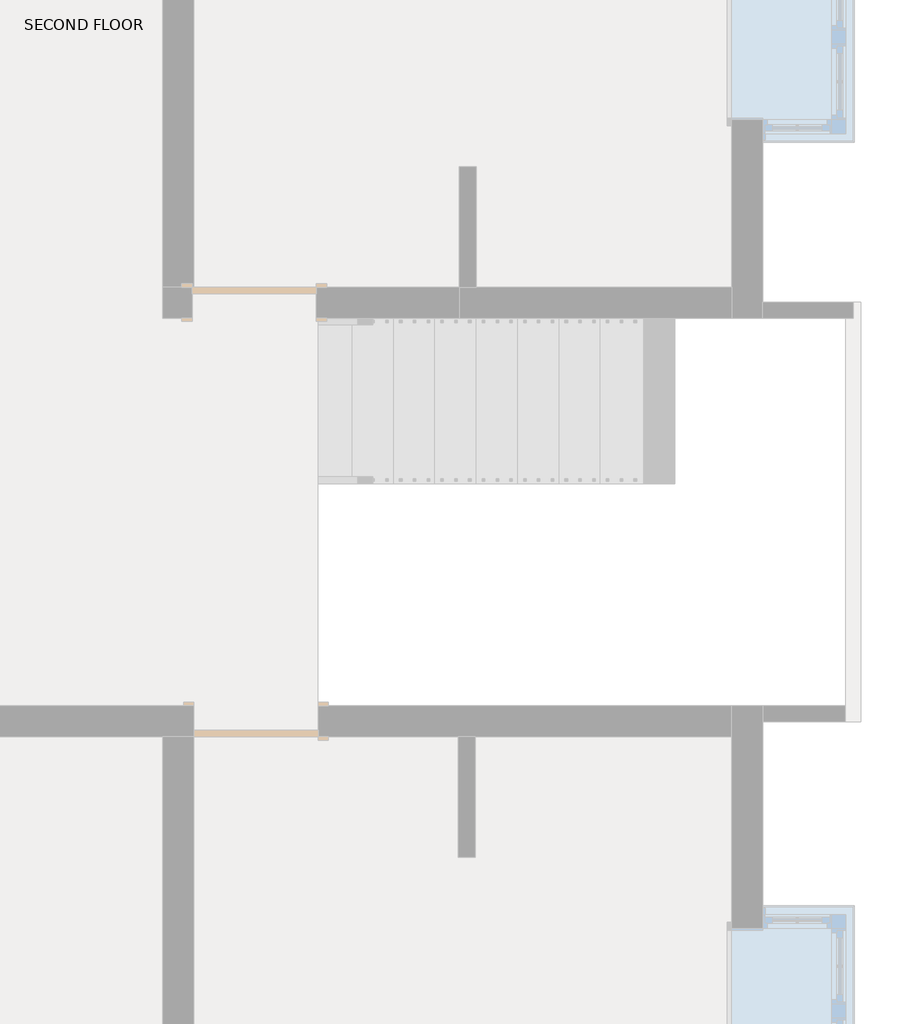
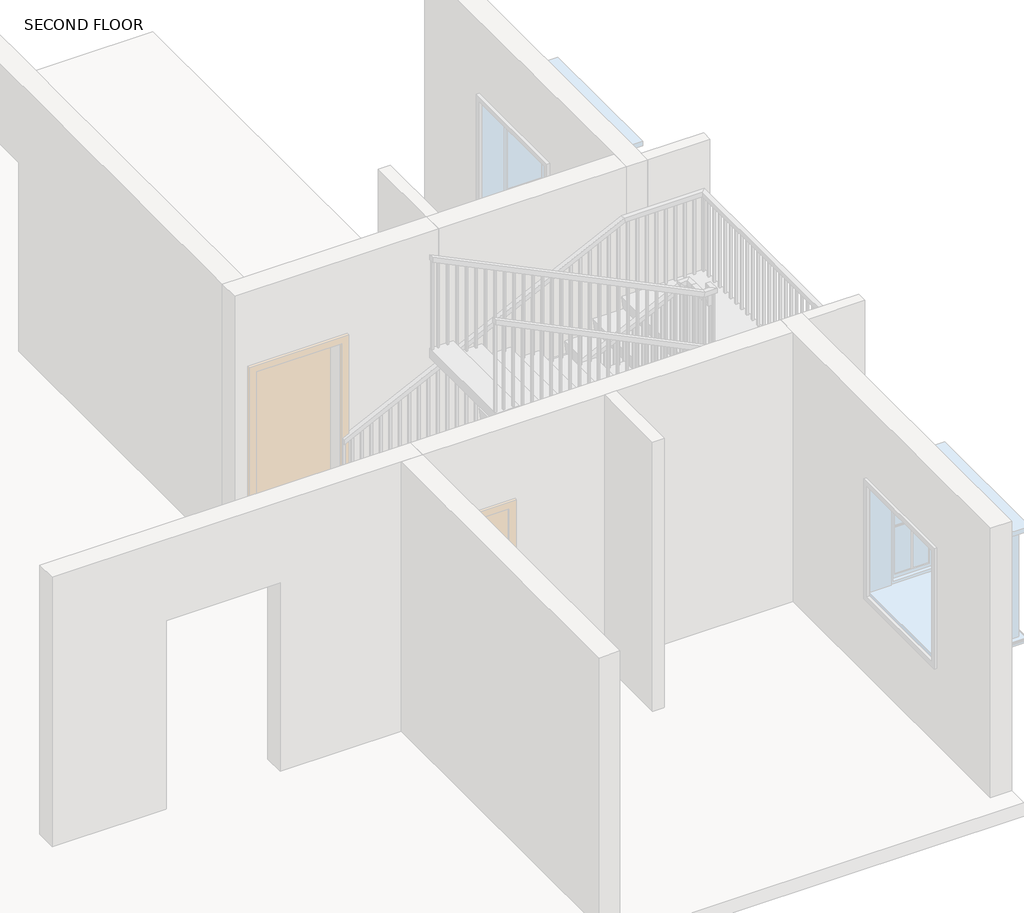
# One storey, part 5 of 6: 1 railing.
"""IFC4 building model written with IfcOpenShell, lengths in millimetres."""

from ifc_helpers import new_model, si_unit, frame, origin, place, context, project, spatial, polyline, outline, extrude, faceted_brep, element, save

model = new_model("IFC4")

# Units and contexts
model_context = context("Model", 3, world=origin())
ifc_project = project(units=[si_unit("LENGTHUNIT", "METRE", prefix="MILLI")], contexts=[model_context])

# Site, building, storey
site = spatial("IfcSite", under=ifc_project)
building = spatial("IfcBuilding", under=site)
storey = spatial("IfcBuildingStorey", under=building, Name="SECOND FLOOR", Elevation=6400.8)

# Railing
placement = place(None, origin())
element("IfcRailing", 1, ObjectType="Handrail - Rectangular", at=placement, inside=storey, context=model_context, shape_type="SolidModel", body=[
    faceted_brep([(3126.2584916, 220.733346, 7460.6727273), (3126.2584916, 220.733346, 7404.1956113), (3126.2584916, 169.933346, 7404.1956113), (3126.2584916, 169.933346, 7460.6727273), (6120.7829507, 220.733346, 8915.4), (6132.4691705, 220.733346, 8864.6), (6132.4691705, 169.933346, 8864.6), (6120.7829507, 169.933346, 8915.4), (7009.1350459, 220.733346, 8915.4), (7009.1350459, 220.733346, 8864.6), (6958.3350459, 169.933346, 8864.6), (6958.3350459, 169.933346, 8915.4), (7009.1350459, -2636.766654, 8915.4), (7009.1350459, -2636.766654, 8864.6), (6958.3350459, -2585.966654, 8864.6), (6958.3350459, -2585.966654, 8915.4), (6420.2353966, -2636.766654, 8915.4), (6408.5491768, -2636.766654, 8864.6), (6408.5491768, -2585.966654, 8864.6), (6420.2353966, -2585.966654, 8915.4), (3126.2584916, -2636.766654, 10515.6), (3126.2584916, -2585.966654, 10515.6), (3126.2584916, -2585.966654, 10459.122884), (3126.2584916, -2636.766654, 10459.122884)], [[[0, 1, 2, 3]], [[1, 0, 4, 5]], [[2, 1, 5, 6]], [[3, 2, 6, 7]], [[0, 3, 7, 4]], [[5, 4, 8, 9]], [[6, 5, 9, 10]], [[7, 6, 10, 11]], [[4, 7, 11, 8]], [[9, 8, 12, 13]], [[10, 9, 13, 14]], [[11, 10, 14, 15]], [[8, 11, 15, 12]], [[13, 12, 16, 17]], [[14, 13, 17, 18]], [[15, 14, 18, 19]], [[12, 15, 19, 16]], [[20, 21, 22, 23]], [[17, 16, 20, 23]], [[18, 17, 23, 22]], [[19, 18, 22, 21]], [[16, 19, 21, 20]]]),
    extrude(outline(polyline([(10416.0077556, 3215.0100459), (9455.7272727, 3215.0100459), (9455.7272727, 3234.0600459), (10406.7533465, 3234.0600459), (10416.0077556, 3215.0100459)])), frame((0.0, -2620.891654, 0.0), z_axis=(0.0, 1.0, 0.0), x_axis=(0.0, 0.0, 1.0)), (0.0, 0.0, 1.0), 19.05),
    extrude(outline(polyline([(10366.6509068, 3316.6100459), (9455.7272727, 3316.6100459), (9455.7272727, 3335.6600459), (10357.3964977, 3335.6600459), (10366.6509068, 3316.6100459)])), frame((0.0, -2620.891654, 0.0), z_axis=(0.0, 1.0, 0.0), x_axis=(0.0, 0.0, 1.0)), (0.0, 0.0, 1.0), 19.05),
    extrude(outline(polyline([(10317.294058, 3418.2100459), (9310.2545455, 3418.2100459), (9310.2545455, 3437.2600459), (10308.0396489, 3437.2600459), (10317.294058, 3418.2100459)])), frame((0.0, -2620.891654, 0.0), z_axis=(0.0, 1.0, 0.0), x_axis=(0.0, 0.0, 1.0)), (0.0, 0.0, 1.0), 19.05),
    extrude(outline(polyline([(10267.9372093, 3519.8100459), (9310.2545455, 3519.8100459), (9310.2545455, 3538.8600459), (10258.6828001, 3538.8600459), (10267.9372093, 3519.8100459)])), frame((0.0, -2620.891654, 0.0), z_axis=(0.0, 1.0, 0.0), x_axis=(0.0, 0.0, 1.0)), (0.0, 0.0, 1.0), 19.05),
    extrude(outline(polyline([(10218.5803605, 3621.4100459), (9310.2545455, 3621.4100459), (9310.2545455, 3640.4600459), (10209.3259513, 3640.4600459), (10218.5803605, 3621.4100459)])), frame((0.0, -2620.891654, 0.0), z_axis=(0.0, 1.0, 0.0), x_axis=(0.0, 0.0, 1.0)), (0.0, 0.0, 1.0), 19.05),
    extrude(outline(polyline([(10169.2235117, 3723.0100459), (9164.7818182, 3723.0100459), (9164.7818182, 3742.0600459), (10159.9691025, 3742.0600459), (10169.2235117, 3723.0100459)])), frame((0.0, -2620.891654, 0.0), z_axis=(0.0, 1.0, 0.0), x_axis=(0.0, 0.0, 1.0)), (0.0, 0.0, 1.0), 19.05),
    extrude(outline(polyline([(10119.8666629, 3824.6100459), (9164.7818182, 3824.6100459), (9164.7818182, 3843.6600459), (10110.6122538, 3843.6600459), (10119.8666629, 3824.6100459)])), frame((0.0, -2620.891654, 0.0), z_axis=(0.0, 1.0, 0.0), x_axis=(0.0, 0.0, 1.0)), (0.0, 0.0, 1.0), 19.05),
    extrude(outline(polyline([(10070.5098141, 3926.2100459), (9164.7818182, 3926.2100459), (9164.7818182, 3945.2600459), (10061.255405, 3945.2600459), (10070.5098141, 3926.2100459)])), frame((0.0, -2620.891654, 0.0), z_axis=(0.0, 1.0, 0.0), x_axis=(0.0, 0.0, 1.0)), (0.0, 0.0, 1.0), 19.05),
    extrude(outline(polyline([(10021.1529653, 4027.8100459), (9019.3090909, 4027.8100459), (9019.3090909, 4046.8600459), (10011.8985562, 4046.8600459), (10021.1529653, 4027.8100459)])), frame((0.0, -2620.891654, 0.0), z_axis=(0.0, 1.0, 0.0), x_axis=(0.0, 0.0, 1.0)), (0.0, 0.0, 1.0), 19.05),
    extrude(outline(polyline([(9971.7961165, 4129.4100459), (9019.3090909, 4129.4100459), (9019.3090909, 4148.4600459), (9962.5417074, 4148.4600459), (9971.7961165, 4129.4100459)])), frame((0.0, -2620.891654, 0.0), z_axis=(0.0, 1.0, 0.0), x_axis=(0.0, 0.0, 1.0)), (0.0, 0.0, 1.0), 19.05),
    extrude(outline(polyline([(9922.4392678, 4231.0100459), (9019.3090909, 4231.0100459), (9019.3090909, 4250.0600459), (9913.1848586, 4250.0600459), (9922.4392678, 4231.0100459)])), frame((0.0, -2620.891654, 0.0), z_axis=(0.0, 1.0, 0.0), x_axis=(0.0, 0.0, 1.0)), (0.0, 0.0, 1.0), 19.05),
    extrude(outline(polyline([(9873.082419, 4332.6100459), (8873.8363636, 4332.6100459), (8873.8363636, 4351.6600459), (9863.8280098, 4351.6600459), (9873.082419, 4332.6100459)])), frame((0.0, -2620.891654, 0.0), z_axis=(0.0, 1.0, 0.0), x_axis=(0.0, 0.0, 1.0)), (0.0, 0.0, 1.0), 19.05),
    extrude(outline(polyline([(9823.7255702, 4434.2100459), (8873.8363636, 4434.2100459), (8873.8363636, 4453.2600459), (9814.471161, 4453.2600459), (9823.7255702, 4434.2100459)])), frame((0.0, -2620.891654, 0.0), z_axis=(0.0, 1.0, 0.0), x_axis=(0.0, 0.0, 1.0)), (0.0, 0.0, 1.0), 19.05),
    extrude(outline(polyline([(9774.3687214, 4535.8100459), (8873.8363636, 4535.8100459), (8873.8363636, 4554.8600459), (9765.1143123, 4554.8600459), (9774.3687214, 4535.8100459)])), frame((0.0, -2620.891654, 0.0), z_axis=(0.0, 1.0, 0.0), x_axis=(0.0, 0.0, 1.0)), (0.0, 0.0, 1.0), 19.05),
    extrude(outline(polyline([(9725.0118726, 4637.4100459), (8728.3636364, 4637.4100459), (8728.3636364, 4656.4600459), (9715.7574635, 4656.4600459), (9725.0118726, 4637.4100459)])), frame((0.0, -2620.891654, 0.0), z_axis=(0.0, 1.0, 0.0), x_axis=(0.0, 0.0, 1.0)), (0.0, 0.0, 1.0), 19.05),
    extrude(outline(polyline([(9675.6550238, 4739.0100459), (8728.3636364, 4739.0100459), (8728.3636364, 4758.0600459), (9666.4006147, 4758.0600459), (9675.6550238, 4739.0100459)])), frame((0.0, -2620.891654, 0.0), z_axis=(0.0, 1.0, 0.0), x_axis=(0.0, 0.0, 1.0)), (0.0, 0.0, 1.0), 19.05),
    extrude(outline(polyline([(9626.2981751, 4840.6100459), (8728.3636364, 4840.6100459), (8728.3636364, 4859.6600459), (9617.0437659, 4859.6600459), (9626.2981751, 4840.6100459)])), frame((0.0, -2620.891654, 0.0), z_axis=(0.0, 1.0, 0.0), x_axis=(0.0, 0.0, 1.0)), (0.0, 0.0, 1.0), 19.05),
    extrude(outline(polyline([(9576.9413263, 4942.2100459), (8582.8909091, 4942.2100459), (8582.8909091, 4961.2600459), (9567.6869171, 4961.2600459), (9576.9413263, 4942.2100459)])), frame((0.0, -2620.891654, 0.0), z_axis=(0.0, 1.0, 0.0), x_axis=(0.0, 0.0, 1.0)), (0.0, 0.0, 1.0), 19.05),
    extrude(outline(polyline([(9527.5844775, 5043.8100459), (8582.8909091, 5043.8100459), (8582.8909091, 5062.8600459), (9518.3300683, 5062.8600459), (9527.5844775, 5043.8100459)])), frame((0.0, -2620.891654, 0.0), z_axis=(0.0, 1.0, 0.0), x_axis=(0.0, 0.0, 1.0)), (0.0, 0.0, 1.0), 19.05),
    extrude(outline(polyline([(9478.2276287, 5145.4100459), (8582.8909091, 5145.4100459), (8582.8909091, 5164.4600459), (9468.9732196, 5164.4600459), (9478.2276287, 5145.4100459)])), frame((0.0, -2620.891654, 0.0), z_axis=(0.0, 1.0, 0.0), x_axis=(0.0, 0.0, 1.0)), (0.0, 0.0, 1.0), 19.05),
    extrude(outline(polyline([(9428.8707799, 5247.0100459), (8437.4181818, 5247.0100459), (8437.4181818, 5266.0600459), (9419.6163708, 5266.0600459), (9428.8707799, 5247.0100459)])), frame((0.0, -2620.891654, 0.0), z_axis=(0.0, 1.0, 0.0), x_axis=(0.0, 0.0, 1.0)), (0.0, 0.0, 1.0), 19.05),
    extrude(outline(polyline([(9379.5139311, 5348.6100459), (8437.4181818, 5348.6100459), (8437.4181818, 5367.6600459), (9370.259522, 5367.6600459), (9379.5139311, 5348.6100459)])), frame((0.0, -2620.891654, 0.0), z_axis=(0.0, 1.0, 0.0), x_axis=(0.0, 0.0, 1.0)), (0.0, 0.0, 1.0), 19.05),
    extrude(outline(polyline([(9330.1570823, 5450.2100459), (8437.4181818, 5450.2100459), (8437.4181818, 5469.2600459), (9320.9026732, 5469.2600459), (9330.1570823, 5450.2100459)])), frame((0.0, -2620.891654, 0.0), z_axis=(0.0, 1.0, 0.0), x_axis=(0.0, 0.0, 1.0)), (0.0, 0.0, 1.0), 19.05),
    extrude(outline(polyline([(9280.8002336, 5551.8100459), (8291.9454545, 5551.8100459), (8291.9454545, 5570.8600459), (9271.5458244, 5570.8600459), (9280.8002336, 5551.8100459)])), frame((0.0, -2620.891654, 0.0), z_axis=(0.0, 1.0, 0.0), x_axis=(0.0, 0.0, 1.0)), (0.0, 0.0, 1.0), 19.05),
    extrude(outline(polyline([(9231.4433848, 5653.4100459), (8291.9454545, 5653.4100459), (8291.9454545, 5672.4600459), (9222.1889756, 5672.4600459), (9231.4433848, 5653.4100459)])), frame((0.0, -2620.891654, 0.0), z_axis=(0.0, 1.0, 0.0), x_axis=(0.0, 0.0, 1.0)), (0.0, 0.0, 1.0), 19.05),
    extrude(outline(polyline([(9182.086536, 5755.0100459), (8291.9454545, 5755.0100459), (8291.9454545, 5774.0600459), (9172.8321268, 5774.0600459), (9182.086536, 5755.0100459)])), frame((0.0, -2620.891654, 0.0), z_axis=(0.0, 1.0, 0.0), x_axis=(0.0, 0.0, 1.0)), (0.0, 0.0, 1.0), 19.05),
    extrude(outline(polyline([(9132.7296872, 5856.6100459), (8146.4727273, 5856.6100459), (8146.4727273, 5875.6600459), (9123.4752781, 5875.6600459), (9132.7296872, 5856.6100459)])), frame((0.0, -2620.891654, 0.0), z_axis=(0.0, 1.0, 0.0), x_axis=(0.0, 0.0, 1.0)), (0.0, 0.0, 1.0), 19.05),
    extrude(outline(polyline([(9083.3728384, 5958.2100459), (8146.4727273, 5958.2100459), (8146.4727273, 5977.2600459), (9074.1184293, 5977.2600459), (9083.3728384, 5958.2100459)])), frame((0.0, -2620.891654, 0.0), z_axis=(0.0, 1.0, 0.0), x_axis=(0.0, 0.0, 1.0)), (0.0, 0.0, 1.0), 19.05),
    extrude(outline(polyline([(9034.0159896, 6059.8100459), (8146.4727273, 6059.8100459), (8146.4727273, 6078.8600459), (9024.7615805, 6078.8600459), (9034.0159896, 6059.8100459)])), frame((0.0, -2620.891654, 0.0), z_axis=(0.0, 1.0, 0.0), x_axis=(0.0, 0.0, 1.0)), (0.0, 0.0, 1.0), 19.05),
    extrude(outline(polyline([(8984.6591409, 6161.4100459), (8001.0, 6161.4100459), (8001.0, 6180.4600459), (8975.4047317, 6180.4600459), (8984.6591409, 6161.4100459)])), frame((0.0, -2620.891654, 0.0), z_axis=(0.0, 1.0, 0.0), x_axis=(0.0, 0.0, 1.0)), (0.0, 0.0, 1.0), 19.05),
    extrude(outline(polyline([(8935.3022921, 6263.0100459), (8001.0, 6263.0100459), (8001.0, 6282.0600459), (8926.0478829, 6282.0600459), (8935.3022921, 6263.0100459)])), frame((0.0, -2620.891654, 0.0), z_axis=(0.0, 1.0, 0.0), x_axis=(0.0, 0.0, 1.0)), (0.0, 0.0, 1.0), 19.05),
    extrude(outline(polyline([(8885.9454433, 6364.6100459), (8001.0, 6364.6100459), (8001.0, 6383.6600459), (8876.6910341, 6383.6600459), (8885.9454433, 6364.6100459)])), frame((0.0, -2620.891654, 0.0), z_axis=(0.0, 1.0, 0.0), x_axis=(0.0, 0.0, 1.0)), (0.0, 0.0, 1.0), 19.05),
    extrude(outline(polyline([(6485.2600459, -2620.891654), (6466.2100459, -2620.891654), (6466.2100459, -2601.841654), (6485.2600459, -2601.841654), (6485.2600459, -2620.891654)])), frame((0.0, 0.0, 8001.0), z_axis=(0.0, 0.0, 1.0), x_axis=(1.0, 0.0, 0.0)), (0.0, 0.0, 1.0), 863.6),
    extrude(outline(polyline([(6586.8600459, -2620.891654), (6567.8100459, -2620.891654), (6567.8100459, -2601.841654), (6586.8600459, -2601.841654), (6586.8600459, -2620.891654)])), frame((0.0, 0.0, 8001.0), z_axis=(0.0, 0.0, 1.0), x_axis=(1.0, 0.0, 0.0)), (0.0, 0.0, 1.0), 863.6),
    extrude(outline(polyline([(6688.4600459, -2620.891654), (6669.4100459, -2620.891654), (6669.4100459, -2601.841654), (6688.4600459, -2601.841654), (6688.4600459, -2620.891654)])), frame((0.0, 0.0, 8001.0), z_axis=(0.0, 0.0, 1.0), x_axis=(1.0, 0.0, 0.0)), (0.0, 0.0, 1.0), 863.6),
    extrude(outline(polyline([(6790.0600459, -2620.891654), (6771.0100459, -2620.891654), (6771.0100459, -2601.841654), (6790.0600459, -2601.841654), (6790.0600459, -2620.891654)])), frame((0.0, 0.0, 8001.0), z_axis=(0.0, 0.0, 1.0), x_axis=(1.0, 0.0, 0.0)), (0.0, 0.0, 1.0), 863.6),
    extrude(outline(polyline([(6891.6600459, -2620.891654), (6872.6100459, -2620.891654), (6872.6100459, -2601.841654), (6891.6600459, -2601.841654), (6891.6600459, -2620.891654)])), frame((0.0, 0.0, 8001.0), z_axis=(0.0, 0.0, 1.0), x_axis=(1.0, 0.0, 0.0)), (0.0, 0.0, 1.0), 863.6),
    extrude(outline(polyline([(6993.2600459, -2538.341654), (6993.2600459, -2557.391654), (6974.2100459, -2557.391654), (6974.2100459, -2538.341654), (6993.2600459, -2538.341654)])), frame((0.0, 0.0, 8001.0), z_axis=(0.0, 0.0, 1.0), x_axis=(1.0, 0.0, 0.0)), (0.0, 0.0, 1.0), 863.6),
    extrude(outline(polyline([(6993.2600459, -2436.741654), (6993.2600459, -2455.791654), (6974.2100459, -2455.791654), (6974.2100459, -2436.741654), (6993.2600459, -2436.741654)])), frame((0.0, 0.0, 8001.0), z_axis=(0.0, 0.0, 1.0), x_axis=(1.0, 0.0, 0.0)), (0.0, 0.0, 1.0), 863.6),
    extrude(outline(polyline([(6993.2600459, -2335.141654), (6993.2600459, -2354.191654), (6974.2100459, -2354.191654), (6974.2100459, -2335.141654), (6993.2600459, -2335.141654)])), frame((0.0, 0.0, 8001.0), z_axis=(0.0, 0.0, 1.0), x_axis=(1.0, 0.0, 0.0)), (0.0, 0.0, 1.0), 863.6),
    extrude(outline(polyline([(6993.2600459, -2233.541654), (6993.2600459, -2252.591654), (6974.2100459, -2252.591654), (6974.2100459, -2233.541654), (6993.2600459, -2233.541654)])), frame((0.0, 0.0, 8001.0), z_axis=(0.0, 0.0, 1.0), x_axis=(1.0, 0.0, 0.0)), (0.0, 0.0, 1.0), 863.6),
    extrude(outline(polyline([(6993.2600459, -2131.941654), (6993.2600459, -2150.991654), (6974.2100459, -2150.991654), (6974.2100459, -2131.941654), (6993.2600459, -2131.941654)])), frame((0.0, 0.0, 8001.0), z_axis=(0.0, 0.0, 1.0), x_axis=(1.0, 0.0, 0.0)), (0.0, 0.0, 1.0), 863.6),
    extrude(outline(polyline([(6993.2600459, -2030.341654), (6993.2600459, -2049.391654), (6974.2100459, -2049.391654), (6974.2100459, -2030.341654), (6993.2600459, -2030.341654)])), frame((0.0, 0.0, 8001.0), z_axis=(0.0, 0.0, 1.0), x_axis=(1.0, 0.0, 0.0)), (0.0, 0.0, 1.0), 863.6),
    extrude(outline(polyline([(6993.2600459, -1928.741654), (6993.2600459, -1947.791654), (6974.2100459, -1947.791654), (6974.2100459, -1928.741654), (6993.2600459, -1928.741654)])), frame((0.0, 0.0, 8001.0), z_axis=(0.0, 0.0, 1.0), x_axis=(1.0, 0.0, 0.0)), (0.0, 0.0, 1.0), 863.6),
    extrude(outline(polyline([(6993.2600459, -1827.141654), (6993.2600459, -1846.191654), (6974.2100459, -1846.191654), (6974.2100459, -1827.141654), (6993.2600459, -1827.141654)])), frame((0.0, 0.0, 8001.0), z_axis=(0.0, 0.0, 1.0), x_axis=(1.0, 0.0, 0.0)), (0.0, 0.0, 1.0), 863.6),
    extrude(outline(polyline([(6993.2600459, -1725.541654), (6993.2600459, -1744.591654), (6974.2100459, -1744.591654), (6974.2100459, -1725.541654), (6993.2600459, -1725.541654)])), frame((0.0, 0.0, 8001.0), z_axis=(0.0, 0.0, 1.0), x_axis=(1.0, 0.0, 0.0)), (0.0, 0.0, 1.0), 863.6),
    extrude(outline(polyline([(6993.2600459, -1623.941654), (6993.2600459, -1642.991654), (6974.2100459, -1642.991654), (6974.2100459, -1623.941654), (6993.2600459, -1623.941654)])), frame((0.0, 0.0, 8001.0), z_axis=(0.0, 0.0, 1.0), x_axis=(1.0, 0.0, 0.0)), (0.0, 0.0, 1.0), 863.6),
    extrude(outline(polyline([(6993.2600459, -1522.341654), (6993.2600459, -1541.391654), (6974.2100459, -1541.391654), (6974.2100459, -1522.341654), (6993.2600459, -1522.341654)])), frame((0.0, 0.0, 8001.0), z_axis=(0.0, 0.0, 1.0), x_axis=(1.0, 0.0, 0.0)), (0.0, 0.0, 1.0), 863.6),
    extrude(outline(polyline([(6993.2600459, -1420.741654), (6993.2600459, -1439.791654), (6974.2100459, -1439.791654), (6974.2100459, -1420.741654), (6993.2600459, -1420.741654)])), frame((0.0, 0.0, 8001.0), z_axis=(0.0, 0.0, 1.0), x_axis=(1.0, 0.0, 0.0)), (0.0, 0.0, 1.0), 863.6),
    extrude(outline(polyline([(6993.2600459, -1319.141654), (6993.2600459, -1338.191654), (6974.2100459, -1338.191654), (6974.2100459, -1319.141654), (6993.2600459, -1319.141654)])), frame((0.0, 0.0, 8001.0), z_axis=(0.0, 0.0, 1.0), x_axis=(1.0, 0.0, 0.0)), (0.0, 0.0, 1.0), 863.6),
    extrude(outline(polyline([(6993.2600459, -1217.541654), (6993.2600459, -1236.591654), (6974.2100459, -1236.591654), (6974.2100459, -1217.541654), (6993.2600459, -1217.541654)])), frame((0.0, 0.0, 8001.0), z_axis=(0.0, 0.0, 1.0), x_axis=(1.0, 0.0, 0.0)), (0.0, 0.0, 1.0), 863.6),
    extrude(outline(polyline([(6993.2600459, -1115.941654), (6993.2600459, -1134.991654), (6974.2100459, -1134.991654), (6974.2100459, -1115.941654), (6993.2600459, -1115.941654)])), frame((0.0, 0.0, 8001.0), z_axis=(0.0, 0.0, 1.0), x_axis=(1.0, 0.0, 0.0)), (0.0, 0.0, 1.0), 863.6),
    extrude(outline(polyline([(6993.2600459, -1014.341654), (6993.2600459, -1033.391654), (6974.2100459, -1033.391654), (6974.2100459, -1014.341654), (6993.2600459, -1014.341654)])), frame((0.0, 0.0, 8001.0), z_axis=(0.0, 0.0, 1.0), x_axis=(1.0, 0.0, 0.0)), (0.0, 0.0, 1.0), 863.6),
    extrude(outline(polyline([(6993.2600459, -912.741654), (6993.2600459, -931.791654), (6974.2100459, -931.791654), (6974.2100459, -912.741654), (6993.2600459, -912.741654)])), frame((0.0, 0.0, 8001.0), z_axis=(0.0, 0.0, 1.0), x_axis=(1.0, 0.0, 0.0)), (0.0, 0.0, 1.0), 863.6),
    extrude(outline(polyline([(6993.2600459, -811.141654), (6993.2600459, -830.191654), (6974.2100459, -830.191654), (6974.2100459, -811.141654), (6993.2600459, -811.141654)])), frame((0.0, 0.0, 8001.0), z_axis=(0.0, 0.0, 1.0), x_axis=(1.0, 0.0, 0.0)), (0.0, 0.0, 1.0), 863.6),
    extrude(outline(polyline([(6993.2600459, -709.541654), (6993.2600459, -728.591654), (6974.2100459, -728.591654), (6974.2100459, -709.541654), (6993.2600459, -709.541654)])), frame((0.0, 0.0, 8001.0), z_axis=(0.0, 0.0, 1.0), x_axis=(1.0, 0.0, 0.0)), (0.0, 0.0, 1.0), 863.6),
    extrude(outline(polyline([(6993.2600459, -607.941654), (6993.2600459, -626.991654), (6974.2100459, -626.991654), (6974.2100459, -607.941654), (6993.2600459, -607.941654)])), frame((0.0, 0.0, 8001.0), z_axis=(0.0, 0.0, 1.0), x_axis=(1.0, 0.0, 0.0)), (0.0, 0.0, 1.0), 863.6),
    extrude(outline(polyline([(6993.2600459, -506.341654), (6993.2600459, -525.391654), (6974.2100459, -525.391654), (6974.2100459, -506.341654), (6993.2600459, -506.341654)])), frame((0.0, 0.0, 8001.0), z_axis=(0.0, 0.0, 1.0), x_axis=(1.0, 0.0, 0.0)), (0.0, 0.0, 1.0), 863.6),
    extrude(outline(polyline([(6993.2600459, -404.741654), (6993.2600459, -423.791654), (6974.2100459, -423.791654), (6974.2100459, -404.741654), (6993.2600459, -404.741654)])), frame((0.0, 0.0, 8001.0), z_axis=(0.0, 0.0, 1.0), x_axis=(1.0, 0.0, 0.0)), (0.0, 0.0, 1.0), 863.6),
    extrude(outline(polyline([(6993.2600459, -303.141654), (6993.2600459, -322.191654), (6974.2100459, -322.191654), (6974.2100459, -303.141654), (6993.2600459, -303.141654)])), frame((0.0, 0.0, 8001.0), z_axis=(0.0, 0.0, 1.0), x_axis=(1.0, 0.0, 0.0)), (0.0, 0.0, 1.0), 863.6),
    extrude(outline(polyline([(6993.2600459, -201.541654), (6993.2600459, -220.591654), (6974.2100459, -220.591654), (6974.2100459, -201.541654), (6993.2600459, -201.541654)])), frame((0.0, 0.0, 8001.0), z_axis=(0.0, 0.0, 1.0), x_axis=(1.0, 0.0, 0.0)), (0.0, 0.0, 1.0), 863.6),
    extrude(outline(polyline([(6993.2600459, -99.941654), (6993.2600459, -118.991654), (6974.2100459, -118.991654), (6974.2100459, -99.941654), (6993.2600459, -99.941654)])), frame((0.0, 0.0, 8001.0), z_axis=(0.0, 0.0, 1.0), x_axis=(1.0, 0.0, 0.0)), (0.0, 0.0, 1.0), 863.6),
    extrude(outline(polyline([(6993.2600459, 1.658346), (6993.2600459, -17.391654), (6974.2100459, -17.391654), (6974.2100459, 1.658346), (6993.2600459, 1.658346)])), frame((0.0, 0.0, 8001.0), z_axis=(0.0, 0.0, 1.0), x_axis=(1.0, 0.0, 0.0)), (0.0, 0.0, 1.0), 863.6),
    extrude(outline(polyline([(6993.2600459, 103.258346), (6993.2600459, 84.208346), (6974.2100459, 84.208346), (6974.2100459, 103.258346), (6993.2600459, 103.258346)])), frame((0.0, 0.0, 8001.0), z_axis=(0.0, 0.0, 1.0), x_axis=(1.0, 0.0, 0.0)), (0.0, 0.0, 1.0), 863.6),
    extrude(outline(polyline([(6875.9334916, 204.858346), (6894.9834916, 204.858346), (6894.9834916, 185.808346), (6875.9334916, 185.808346), (6875.9334916, 204.858346)])), frame((0.0, 0.0, 8001.0), z_axis=(0.0, 0.0, 1.0), x_axis=(1.0, 0.0, 0.0)), (0.0, 0.0, 1.0), 863.6),
    extrude(outline(polyline([(6774.3334916, 204.858346), (6793.3834916, 204.858346), (6793.3834916, 185.808346), (6774.3334916, 185.808346), (6774.3334916, 204.858346)])), frame((0.0, 0.0, 8001.0), z_axis=(0.0, 0.0, 1.0), x_axis=(1.0, 0.0, 0.0)), (0.0, 0.0, 1.0), 863.6),
    extrude(outline(polyline([(6672.7334916, 204.858346), (6691.7834916, 204.858346), (6691.7834916, 185.808346), (6672.7334916, 185.808346), (6672.7334916, 204.858346)])), frame((0.0, 0.0, 8001.0), z_axis=(0.0, 0.0, 1.0), x_axis=(1.0, 0.0, 0.0)), (0.0, 0.0, 1.0), 863.6),
    extrude(outline(polyline([(6571.1334916, 204.858346), (6590.1834916, 204.858346), (6590.1834916, 185.808346), (6571.1334916, 185.808346), (6571.1334916, 204.858346)])), frame((0.0, 0.0, 8001.0), z_axis=(0.0, 0.0, 1.0), x_axis=(1.0, 0.0, 0.0)), (0.0, 0.0, 1.0), 863.6),
    extrude(outline(polyline([(6469.5334916, 204.858346), (6488.5834916, 204.858346), (6488.5834916, 185.808346), (6469.5334916, 185.808346), (6469.5334916, 204.858346)])), frame((0.0, 0.0, 8001.0), z_axis=(0.0, 0.0, 1.0), x_axis=(1.0, 0.0, 0.0)), (0.0, 0.0, 1.0), 863.6),
    extrude(outline(polyline([(6367.9334916, 204.858346), (6386.9834916, 204.858346), (6386.9834916, 185.808346), (6367.9334916, 185.808346), (6367.9334916, 204.858346)])), frame((0.0, 0.0, 8001.0), z_axis=(0.0, 0.0, 1.0), x_axis=(1.0, 0.0, 0.0)), (0.0, 0.0, 1.0), 863.6),
    extrude(outline(polyline([(6266.3334916, 204.858346), (6285.3834916, 204.858346), (6285.3834916, 185.808346), (6266.3334916, 185.808346), (6266.3334916, 204.858346)])), frame((0.0, 0.0, 8001.0), z_axis=(0.0, 0.0, 1.0), x_axis=(1.0, 0.0, 0.0)), (0.0, 0.0, 1.0), 863.6),
    extrude(outline(polyline([(6164.7334916, 204.858346), (6183.7834916, 204.858346), (6183.7834916, 185.808346), (6164.7334916, 185.808346), (6164.7334916, 204.858346)])), frame((0.0, 0.0, 8001.0), z_axis=(0.0, 0.0, 1.0), x_axis=(1.0, 0.0, 0.0)), (0.0, 0.0, 1.0), 863.6),
    extrude(outline(polyline([(8830.9170215, 6063.1334916), (7855.5272727, 6063.1334916), (7855.5272727, 6082.1834916), (8840.1714306, 6082.1834916), (8830.9170215, 6063.1334916)])), frame((0.0, 185.808346, 0.0), z_axis=(0.0, 1.0, 0.0), x_axis=(0.0, 0.0, 1.0)), (0.0, 0.0, 1.0), 19.05),
    extrude(outline(polyline([(8781.5601727, 5961.5334916), (7855.5272727, 5961.5334916), (7855.5272727, 5980.5834916), (8790.8145818, 5980.5834916), (8781.5601727, 5961.5334916)])), frame((0.0, 185.808346, 0.0), z_axis=(0.0, 1.0, 0.0), x_axis=(0.0, 0.0, 1.0)), (0.0, 0.0, 1.0), 19.05),
    extrude(outline(polyline([(8732.2033239, 5859.9334916), (7855.5272727, 5859.9334916), (7855.5272727, 5878.9834916), (8741.457733, 5878.9834916), (8732.2033239, 5859.9334916)])), frame((0.0, 185.808346, 0.0), z_axis=(0.0, 1.0, 0.0), x_axis=(0.0, 0.0, 1.0)), (0.0, 0.0, 1.0), 19.05),
    extrude(outline(polyline([(8682.8464751, 5758.3334916), (7710.0545455, 5758.3334916), (7710.0545455, 5777.3834916), (8692.1008843, 5777.3834916), (8682.8464751, 5758.3334916)])), frame((0.0, 185.808346, 0.0), z_axis=(0.0, 1.0, 0.0), x_axis=(0.0, 0.0, 1.0)), (0.0, 0.0, 1.0), 19.05),
    extrude(outline(polyline([(8633.4896263, 5656.7334916), (7710.0545455, 5656.7334916), (7710.0545455, 5675.7834916), (8642.7440355, 5675.7834916), (8633.4896263, 5656.7334916)])), frame((0.0, 185.808346, 0.0), z_axis=(0.0, 1.0, 0.0), x_axis=(0.0, 0.0, 1.0)), (0.0, 0.0, 1.0), 19.05),
    extrude(outline(polyline([(8584.1327775, 5555.1334916), (7710.0545455, 5555.1334916), (7710.0545455, 5574.1834916), (8593.3871867, 5574.1834916), (8584.1327775, 5555.1334916)])), frame((0.0, 185.808346, 0.0), z_axis=(0.0, 1.0, 0.0), x_axis=(0.0, 0.0, 1.0)), (0.0, 0.0, 1.0), 19.05),
    extrude(outline(polyline([(8534.7759288, 5453.5334916), (7564.5818182, 5453.5334916), (7564.5818182, 5472.5834916), (8544.0303379, 5472.5834916), (8534.7759288, 5453.5334916)])), frame((0.0, 185.808346, 0.0), z_axis=(0.0, 1.0, 0.0), x_axis=(0.0, 0.0, 1.0)), (0.0, 0.0, 1.0), 19.05),
    extrude(outline(polyline([(8485.41908, 5351.9334916), (7564.5818182, 5351.9334916), (7564.5818182, 5370.9834916), (8494.6734891, 5370.9834916), (8485.41908, 5351.9334916)])), frame((0.0, 185.808346, 0.0), z_axis=(0.0, 1.0, 0.0), x_axis=(0.0, 0.0, 1.0)), (0.0, 0.0, 1.0), 19.05),
    extrude(outline(polyline([(8436.0622312, 5250.3334916), (7564.5818182, 5250.3334916), (7564.5818182, 5269.3834916), (8445.3166403, 5269.3834916), (8436.0622312, 5250.3334916)])), frame((0.0, 185.808346, 0.0), z_axis=(0.0, 1.0, 0.0), x_axis=(0.0, 0.0, 1.0)), (0.0, 0.0, 1.0), 19.05),
    extrude(outline(polyline([(8386.7053824, 5148.7334916), (7419.1090909, 5148.7334916), (7419.1090909, 5167.7834916), (8395.9597915, 5167.7834916), (8386.7053824, 5148.7334916)])), frame((0.0, 185.808346, 0.0), z_axis=(0.0, 1.0, 0.0), x_axis=(0.0, 0.0, 1.0)), (0.0, 0.0, 1.0), 19.05),
    extrude(outline(polyline([(8337.3485336, 5047.1334916), (7419.1090909, 5047.1334916), (7419.1090909, 5066.1834916), (8346.6029428, 5066.1834916), (8337.3485336, 5047.1334916)])), frame((0.0, 185.808346, 0.0), z_axis=(0.0, 1.0, 0.0), x_axis=(0.0, 0.0, 1.0)), (0.0, 0.0, 1.0), 19.05),
    extrude(outline(polyline([(8287.9916848, 4945.5334916), (7419.1090909, 4945.5334916), (7419.1090909, 4964.5834916), (8297.246094, 4964.5834916), (8287.9916848, 4945.5334916)])), frame((0.0, 185.808346, 0.0), z_axis=(0.0, 1.0, 0.0), x_axis=(0.0, 0.0, 1.0)), (0.0, 0.0, 1.0), 19.05),
    extrude(outline(polyline([(8238.634836, 4843.9334916), (7273.6363636, 4843.9334916), (7273.6363636, 4862.9834916), (8247.8892452, 4862.9834916), (8238.634836, 4843.9334916)])), frame((0.0, 185.808346, 0.0), z_axis=(0.0, 1.0, 0.0), x_axis=(0.0, 0.0, 1.0)), (0.0, 0.0, 1.0), 19.05),
    extrude(outline(polyline([(8189.2779873, 4742.3334916), (7273.6363636, 4742.3334916), (7273.6363636, 4761.3834916), (8198.5323964, 4761.3834916), (8189.2779873, 4742.3334916)])), frame((0.0, 185.808346, 0.0), z_axis=(0.0, 1.0, 0.0), x_axis=(0.0, 0.0, 1.0)), (0.0, 0.0, 1.0), 19.05),
    extrude(outline(polyline([(8139.9211385, 4640.7334916), (7273.6363636, 4640.7334916), (7273.6363636, 4659.7834916), (8149.1755476, 4659.7834916), (8139.9211385, 4640.7334916)])), frame((0.0, 185.808346, 0.0), z_axis=(0.0, 1.0, 0.0), x_axis=(0.0, 0.0, 1.0)), (0.0, 0.0, 1.0), 19.05),
    extrude(outline(polyline([(8090.5642897, 4539.1334916), (7128.1636364, 4539.1334916), (7128.1636364, 4558.1834916), (8099.8186988, 4558.1834916), (8090.5642897, 4539.1334916)])), frame((0.0, 185.808346, 0.0), z_axis=(0.0, 1.0, 0.0), x_axis=(0.0, 0.0, 1.0)), (0.0, 0.0, 1.0), 19.05),
    extrude(outline(polyline([(8041.2074409, 4437.5334916), (7128.1636364, 4437.5334916), (7128.1636364, 4456.5834916), (8050.4618501, 4456.5834916), (8041.2074409, 4437.5334916)])), frame((0.0, 185.808346, 0.0), z_axis=(0.0, 1.0, 0.0), x_axis=(0.0, 0.0, 1.0)), (0.0, 0.0, 1.0), 19.05),
    extrude(outline(polyline([(7991.8505921, 4335.9334916), (7128.1636364, 4335.9334916), (7128.1636364, 4354.9834916), (8001.1050013, 4354.9834916), (7991.8505921, 4335.9334916)])), frame((0.0, 185.808346, 0.0), z_axis=(0.0, 1.0, 0.0), x_axis=(0.0, 0.0, 1.0)), (0.0, 0.0, 1.0), 19.05),
    extrude(outline(polyline([(7942.4937433, 4234.3334916), (6982.6909091, 4234.3334916), (6982.6909091, 4253.3834916), (7951.7481525, 4253.3834916), (7942.4937433, 4234.3334916)])), frame((0.0, 185.808346, 0.0), z_axis=(0.0, 1.0, 0.0), x_axis=(0.0, 0.0, 1.0)), (0.0, 0.0, 1.0), 19.05),
    extrude(outline(polyline([(7893.1368946, 4132.7334916), (6982.6909091, 4132.7334916), (6982.6909091, 4151.7834916), (7902.3913037, 4151.7834916), (7893.1368946, 4132.7334916)])), frame((0.0, 185.808346, 0.0), z_axis=(0.0, 1.0, 0.0), x_axis=(0.0, 0.0, 1.0)), (0.0, 0.0, 1.0), 19.05),
    extrude(outline(polyline([(7843.7800458, 4031.1334916), (6982.6909091, 4031.1334916), (6982.6909091, 4050.1834916), (7853.0344549, 4050.1834916), (7843.7800458, 4031.1334916)])), frame((0.0, 185.808346, 0.0), z_axis=(0.0, 1.0, 0.0), x_axis=(0.0, 0.0, 1.0)), (0.0, 0.0, 1.0), 19.05),
    extrude(outline(polyline([(7794.423197, 3929.5334916), (6837.2181818, 3929.5334916), (6837.2181818, 3948.5834916), (7803.6776061, 3948.5834916), (7794.423197, 3929.5334916)])), frame((0.0, 185.808346, 0.0), z_axis=(0.0, 1.0, 0.0), x_axis=(0.0, 0.0, 1.0)), (0.0, 0.0, 1.0), 19.05),
    extrude(outline(polyline([(7745.0663482, 3827.9334916), (6837.2181818, 3827.9334916), (6837.2181818, 3846.9834916), (7754.3207573, 3846.9834916), (7745.0663482, 3827.9334916)])), frame((0.0, 185.808346, 0.0), z_axis=(0.0, 1.0, 0.0), x_axis=(0.0, 0.0, 1.0)), (0.0, 0.0, 1.0), 19.05),
    extrude(outline(polyline([(7695.7094994, 3726.3334916), (6837.2181818, 3726.3334916), (6837.2181818, 3745.3834916), (7704.9639086, 3745.3834916), (7695.7094994, 3726.3334916)])), frame((0.0, 185.808346, 0.0), z_axis=(0.0, 1.0, 0.0), x_axis=(0.0, 0.0, 1.0)), (0.0, 0.0, 1.0), 19.05),
    extrude(outline(polyline([(7646.3526506, 3624.7334916), (6691.7454545, 3624.7334916), (6691.7454545, 3643.7834916), (7655.6070598, 3643.7834916), (7646.3526506, 3624.7334916)])), frame((0.0, 185.808346, 0.0), z_axis=(0.0, 1.0, 0.0), x_axis=(0.0, 0.0, 1.0)), (0.0, 0.0, 1.0), 19.05),
    extrude(outline(polyline([(7596.9958018, 3523.1334916), (6691.7454545, 3523.1334916), (6691.7454545, 3542.1834916), (7606.250211, 3542.1834916), (7596.9958018, 3523.1334916)])), frame((0.0, 185.808346, 0.0), z_axis=(0.0, 1.0, 0.0), x_axis=(0.0, 0.0, 1.0)), (0.0, 0.0, 1.0), 19.05),
    extrude(outline(polyline([(7547.6389531, 3421.5334916), (6691.7454545, 3421.5334916), (6691.7454545, 3440.5834916), (7556.8933622, 3440.5834916), (7547.6389531, 3421.5334916)])), frame((0.0, 185.808346, 0.0), z_axis=(0.0, 1.0, 0.0), x_axis=(0.0, 0.0, 1.0)), (0.0, 0.0, 1.0), 19.05),
    extrude(outline(polyline([(7498.2821043, 3319.9334916), (6546.2727273, 3319.9334916), (6546.2727273, 3338.9834916), (7507.5365134, 3338.9834916), (7498.2821043, 3319.9334916)])), frame((0.0, 185.808346, 0.0), z_axis=(0.0, 1.0, 0.0), x_axis=(0.0, 0.0, 1.0)), (0.0, 0.0, 1.0), 19.05),
    extrude(outline(polyline([(7448.9252555, 3218.3334916), (6546.2727273, 3218.3334916), (6546.2727273, 3237.3834916), (7458.1796646, 3237.3834916), (7448.9252555, 3218.3334916)])), frame((0.0, 185.808346, 0.0), z_axis=(0.0, 1.0, 0.0), x_axis=(0.0, 0.0, 1.0)), (0.0, 0.0, 1.0), 19.05),
    extrude(outline(polyline([(6993.2600459, -2601.841654), (6993.2600459, -2620.891654), (6974.2100459, -2620.891654), (6974.2100459, -2601.841654), (6993.2600459, -2601.841654)])), frame((0.0, 0.0, 8001.0), z_axis=(0.0, 0.0, 1.0), x_axis=(1.0, 0.0, 0.0)), (0.0, 0.0, 1.0), 863.6),
    extrude(outline(polyline([(6974.2100459, 204.858346), (6993.2600459, 204.858346), (6993.2600459, 185.808346), (6974.2100459, 185.808346), (6974.2100459, 204.858346)])), frame((0.0, 0.0, 8001.0), z_axis=(0.0, 0.0, 1.0), x_axis=(1.0, 0.0, 0.0)), (0.0, 0.0, 1.0), 863.6),
    extrude(outline(polyline([(10459.122884, 3126.2584916), (9455.7272727, 3126.2584916), (9455.7272727, 3145.3084916), (10449.8684749, 3145.3084916), (10459.122884, 3126.2584916)])), frame((0.0, -2620.891654, 0.0), z_axis=(0.0, 1.0, 0.0), x_axis=(0.0, 0.0, 1.0)), (0.0, 0.0, 1.0), 19.05),
    extrude(outline(polyline([(7404.1956113, 3126.2584916), (6546.2727273, 3126.2584916), (6546.2727273, 3145.3084916), (7413.4500204, 3145.3084916), (7404.1956113, 3126.2584916)])), frame((0.0, 185.808346, 0.0), z_axis=(0.0, 1.0, 0.0), x_axis=(0.0, 0.0, 1.0)), (0.0, 0.0, 1.0), 19.05),
])

save(model, "model.ifc")

# Revit data of these elements
# Type "Handrail - Rectangular"
#   Assembly Code = "C2010400"
#   built-in parameter 1008612 = 0.0416667 (stored number, unit not read)
#   built-in parameter 1008611 = 0.0416667 (stored number, unit not read)
#   built-in parameter 1008609 = 0.333333 (stored number, unit not read)
#   built-in parameter 1008604 = 0.166667 (stored number, unit not read)
#   built-in parameter 1008603 = 0.166667 (stored number, unit not read)
#   Railing Height = 3' - 0"
#   built-in parameter 1008630 = 2
#   built-in parameter 1008610 = 2
#   built-in parameter 1008618 = Baluster - Square : 3/4"
# Element 1 (IfcRailing, "Handrail - Rectangular")
#   Phase Created = New Construction
